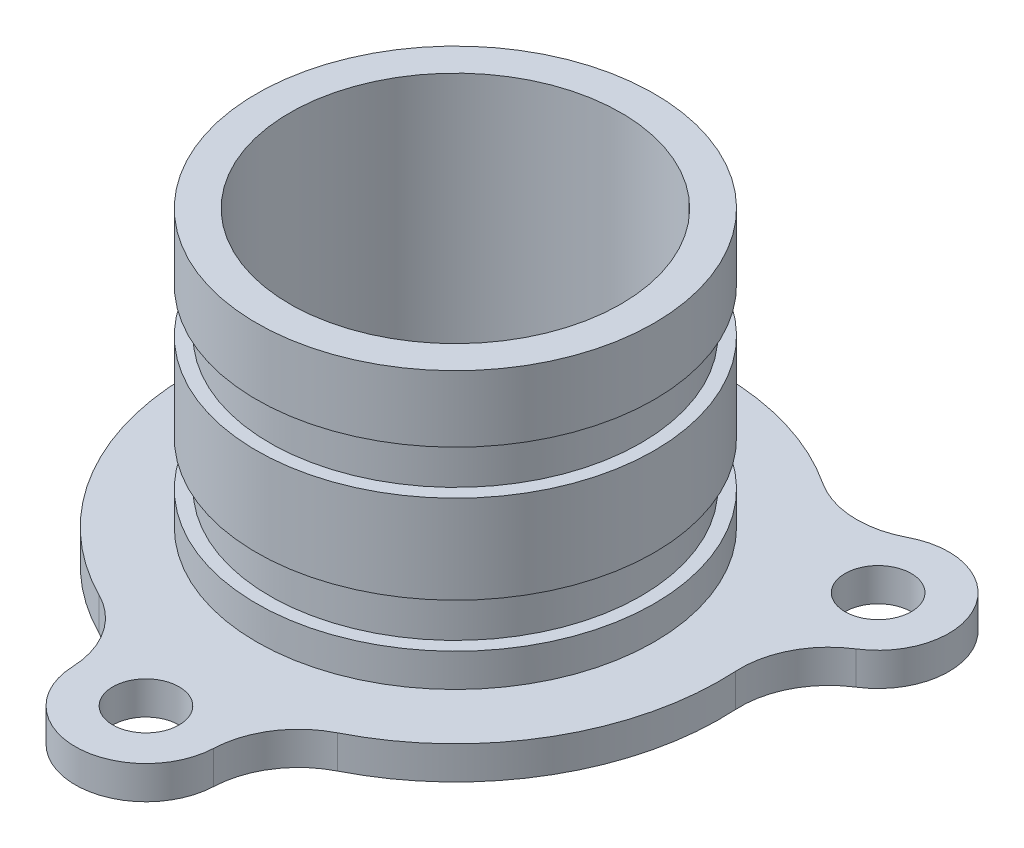
ISO-10303-21;
HEADER;
FILE_DESCRIPTION(('STEP AP214'),'2;1');
FILE_NAME('part.step','',(''),(''),'','','');
FILE_SCHEMA(('AUTOMOTIVE_DESIGN { 1 0 10303 214 1 1 1 1 }'));
ENDSEC;
DATA;
#1=APPLICATION_CONTEXT('core data for automotive mechanical design processes');
#2=APPLICATION_PROTOCOL_DEFINITION('international standard','automotive_design',2000,#1);
#3=PRODUCT_CONTEXT('',#1,'mechanical');
#4=PRODUCT('Part','Part','',(#3));
#5=PRODUCT_RELATED_PRODUCT_CATEGORY('part','',(#4));
#6=PRODUCT_DEFINITION_FORMATION('','',#4);
#7=PRODUCT_DEFINITION_CONTEXT('part definition',#1,'design');
#8=PRODUCT_DEFINITION('design','',#6,#7);
#9=PRODUCT_DEFINITION_SHAPE('','',#8);
#10=(LENGTH_UNIT() NAMED_UNIT(*) SI_UNIT(.MILLI.,.METRE.));
#11=(NAMED_UNIT(*) PLANE_ANGLE_UNIT() SI_UNIT($,.RADIAN.));
#12=(NAMED_UNIT(*) SI_UNIT($,.STERADIAN.) SOLID_ANGLE_UNIT());
#13=UNCERTAINTY_MEASURE_WITH_UNIT(LENGTH_MEASURE(1.E-05),#10,'distance_accuracy_value','');
#14=(GEOMETRIC_REPRESENTATION_CONTEXT(3) GLOBAL_UNCERTAINTY_ASSIGNED_CONTEXT((#13)) GLOBAL_UNIT_ASSIGNED_CONTEXT((#10,
#11,#12)) REPRESENTATION_CONTEXT('',''));
#15=CARTESIAN_POINT('',(0.,0.,0.));
#16=DIRECTION('',(0.,0.,1.));
#17=DIRECTION('',(1.,0.,0.));
#18=AXIS2_PLACEMENT_3D('',#15,#16,#17);
#19=CARTESIAN_POINT('',(45.,70.,0.));
#20=DIRECTION('',(0.,1.,0.));
#21=DIRECTION('',(-1.,0.,0.));
#22=AXIS2_PLACEMENT_3D('',#19,#20,#21);
#23=PLANE('',#22);
#24=CARTESIAN_POINT('',(0.,70.,0.));
#25=DIRECTION('',(0.,-1.,0.));
#26=DIRECTION('',(1.,0.,0.));
#27=AXIS2_PLACEMENT_3D('',#24,#25,#26);
#28=CIRCLE('',#27,37.5);
#29=CARTESIAN_POINT('',(37.5,70.,0.));
#30=VERTEX_POINT('',#29);
#31=EDGE_CURVE('E50',#30,#30,#28,.T.);
#32=ORIENTED_EDGE('',*,*,#31,.T.);
#33=EDGE_LOOP('',(#32));
#34=FACE_BOUND('',#33,.T.);
#35=CARTESIAN_POINT('',(0.,70.,0.));
#36=DIRECTION('',(0.,-1.,0.));
#37=DIRECTION('',(1.,0.,0.));
#38=AXIS2_PLACEMENT_3D('',#35,#36,#37);
#39=CIRCLE('',#38,45.);
#40=CARTESIAN_POINT('',(45.,70.,0.));
#41=VERTEX_POINT('',#40);
#42=EDGE_CURVE('E196',#41,#41,#39,.T.);
#43=ORIENTED_EDGE('',*,*,#42,.F.);
#44=EDGE_LOOP('',(#43));
#45=FACE_BOUND('',#44,.T.);
#46=ADVANCED_FACE('F39',(#34,#45),#23,.T.);
#47=CARTESIAN_POINT('',(0.,-100.894385011522,0.));
#48=DIRECTION('',(0.,-1.,0.));
#49=DIRECTION('',(1.,0.,0.));
#50=AXIS2_PLACEMENT_3D('',#47,#48,#49);
#51=CYLINDRICAL_SURFACE('',#50,37.5);
#52=ORIENTED_EDGE('',*,*,#31,.F.);
#53=EDGE_LOOP('',(#52));
#54=FACE_BOUND('',#53,.T.);
#55=CARTESIAN_POINT('',(0.,0.,0.));
#56=DIRECTION('',(0.,-1.,0.));
#57=DIRECTION('',(1.,0.,0.));
#58=AXIS2_PLACEMENT_3D('',#55,#56,#57);
#59=CIRCLE('',#58,37.5);
#60=CARTESIAN_POINT('',(37.5,0.,0.));
#61=VERTEX_POINT('',#60);
#62=EDGE_CURVE('E244',#61,#61,#59,.T.);
#63=ORIENTED_EDGE('',*,*,#62,.T.);
#64=EDGE_LOOP('',(#63));
#65=FACE_BOUND('',#64,.T.);
#66=ADVANCED_FACE('F247',(#54,#65),#51,.F.);
#67=CARTESIAN_POINT('',(45.,0.,0.));
#68=DIRECTION('',(0.,-1.,0.));
#69=DIRECTION('',(1.,0.,0.));
#70=AXIS2_PLACEMENT_3D('',#67,#68,#69);
#71=PLANE('',#70);
#72=ORIENTED_EDGE('',*,*,#62,.F.);
#73=EDGE_LOOP('',(#72));
#74=FACE_BOUND('',#73,.T.);
#75=CARTESIAN_POINT('',(-60.6650795351003,0.,-35.0249999999994));
#76=DIRECTION('',(0.,-1.,0.));
#77=DIRECTION('',(1.,0.,0.));
#78=AXIS2_PLACEMENT_3D('',#75,#76,#77);
#79=CIRCLE('',#78,7.5);
#80=CARTESIAN_POINT('',(-53.1650795351003,0.,-35.0249999999994));
#81=VERTEX_POINT('',#80);
#82=EDGE_CURVE('E265',#81,#81,#79,.T.);
#83=ORIENTED_EDGE('',*,*,#82,.F.);
#84=EDGE_LOOP('',(#83));
#85=FACE_BOUND('',#84,.T.);
#86=CARTESIAN_POINT('',(60.6650795350998,0.,-35.0250000000003));
#87=DIRECTION('',(0.,-1.,0.));
#88=DIRECTION('',(1.,0.,0.));
#89=AXIS2_PLACEMENT_3D('',#86,#87,#88);
#90=CIRCLE('',#89,7.50000000000001);
#91=CARTESIAN_POINT('',(68.1650795350998,0.,-35.0250000000003));
#92=VERTEX_POINT('',#91);
#93=EDGE_CURVE('E266',#92,#92,#90,.T.);
#94=ORIENTED_EDGE('',*,*,#93,.F.);
#95=EDGE_LOOP('',(#94));
#96=FACE_BOUND('',#95,.T.);
#97=CARTESIAN_POINT('',(0.,0.,70.05));
#98=DIRECTION('',(0.,-1.,0.));
#99=DIRECTION('',(1.,0.,0.));
#100=AXIS2_PLACEMENT_3D('',#97,#98,#99);
#101=CIRCLE('',#100,7.5);
#102=CARTESIAN_POINT('',(7.5,0.,70.05));
#103=VERTEX_POINT('',#102);
#104=EDGE_CURVE('E269',#103,#103,#101,.T.);
#105=ORIENTED_EDGE('',*,*,#104,.F.);
#106=EDGE_LOOP('',(#105));
#107=FACE_BOUND('',#106,.T.);
#108=CARTESIAN_POINT('',(-35.9702505845438,0.,71.5132405424697));
#109=DIRECTION('',(0.,1.,0.));
#110=DIRECTION('',(-1.,0.,0.));
#111=AXIS2_PLACEMENT_3D('',#108,#109,#110);
#112=CIRCLE('',#111,20.);
#113=CARTESIAN_POINT('',(-15.986778037575,0.,70.7003291299865));
#114=VERTEX_POINT('',#113);
#115=CARTESIAN_POINT('',(-26.983304779536,0.,53.6460973713342));
#116=VERTEX_POINT('',#115);
#117=EDGE_CURVE('E165',#114,#116,#112,.T.);
#118=ORIENTED_EDGE('',*,*,#117,.T.);
#119=CARTESIAN_POINT('',(0.,0.,0.));
#120=DIRECTION('',(0.,-1.,0.));
#121=DIRECTION('',(1.,0.,0.));
#122=AXIS2_PLACEMENT_3D('',#119,#120,#121);
#123=CIRCLE('',#122,60.05);
#124=CARTESIAN_POINT('',(-59.950535527237,0.,-3.45482126853093));
#125=VERTEX_POINT('',#124);
#126=EDGE_CURVE('E164',#116,#125,#123,.T.);
#127=ORIENTED_EDGE('',*,*,#126,.T.);
#128=CARTESIAN_POINT('',(-79.9174083089979,0.,-4.60546948452791));
#129=DIRECTION('',(0.,1.,0.));
#130=DIRECTION('',(1.,0.,0.));
#131=AXIS2_PLACEMENT_3D('',#128,#129,#130);
#132=CIRCLE('',#131,20.);
#133=CARTESIAN_POINT('',(-69.2216701012772,0.,-21.5052086597896));
#134=VERTEX_POINT('',#133);
#135=EDGE_CURVE('E166',#125,#134,#132,.T.);
#136=ORIENTED_EDGE('',*,*,#135,.T.);
#137=CARTESIAN_POINT('',(-60.6650795351003,0.,-35.0249999999994));
#138=DIRECTION('',(0.,-1.,0.));
#139=DIRECTION('',(1.,0.,0.));
#140=AXIS2_PLACEMENT_3D('',#137,#138,#139);
#141=CIRCLE('',#140,16.);
#142=CARTESIAN_POINT('',(-53.2348920637018,0.,-49.1951204701964));
#143=VERTEX_POINT('',#142);
#144=EDGE_CURVE('E174',#134,#143,#141,.T.);
#145=ORIENTED_EDGE('',*,*,#144,.T.);
#146=CARTESIAN_POINT('',(-43.9471577244541,0.,-66.9077710579418));
#147=DIRECTION('',(0.,1.,0.));
#148=DIRECTION('',(-1.,0.,0.));
#149=AXIS2_PLACEMENT_3D('',#146,#147,#148);
#150=CIRCLE('',#149,20.);
#151=CARTESIAN_POINT('',(-32.9672307477011,0.,-50.1912761028033));
#152=VERTEX_POINT('',#151);
#153=EDGE_CURVE('E171',#143,#152,#150,.T.);
#154=ORIENTED_EDGE('',*,*,#153,.T.);
#155=CARTESIAN_POINT('',(0.,0.,0.));
#156=DIRECTION('',(0.,-1.,0.));
#157=DIRECTION('',(1.,0.,0.));
#158=AXIS2_PLACEMENT_3D('',#155,#156,#157);
#159=CIRCLE('',#158,60.05);
#160=CARTESIAN_POINT('',(32.9672307477011,0.,-50.1912761028033));
#161=VERTEX_POINT('',#160);
#162=EDGE_CURVE('E178',#152,#161,#159,.T.);
#163=ORIENTED_EDGE('',*,*,#162,.T.);
#164=CARTESIAN_POINT('',(43.9471577244538,0.,-66.907771057942));
#165=DIRECTION('',(0.,1.,0.));
#166=DIRECTION('',(1.,0.,0.));
#167=AXIS2_PLACEMENT_3D('',#164,#165,#166);
#168=CIRCLE('',#167,20.);
#169=CARTESIAN_POINT('',(53.2348920637016,0.,-49.1951204701966));
#170=VERTEX_POINT('',#169);
#171=EDGE_CURVE('E182',#161,#170,#168,.T.);
#172=ORIENTED_EDGE('',*,*,#171,.T.);
#173=CARTESIAN_POINT('',(60.6650795350998,0.,-35.0250000000003));
#174=DIRECTION('',(0.,-1.,0.));
#175=DIRECTION('',(1.,0.,0.));
#176=AXIS2_PLACEMENT_3D('',#173,#174,#175);
#177=CIRCLE('',#176,16.);
#178=CARTESIAN_POINT('',(69.2216701012767,0.,-21.5052086597905));
#179=VERTEX_POINT('',#178);
#180=EDGE_CURVE('E184',#170,#179,#177,.T.);
#181=ORIENTED_EDGE('',*,*,#180,.T.);
#182=CARTESIAN_POINT('',(79.9174083089979,0.,-4.60546948452819));
#183=DIRECTION('',(0.,1.,0.));
#184=DIRECTION('',(-1.,0.,0.));
#185=AXIS2_PLACEMENT_3D('',#182,#183,#184);
#186=CIRCLE('',#185,20.);
#187=CARTESIAN_POINT('',(59.950535527237,0.,-3.45482126853086));
#188=VERTEX_POINT('',#187);
#189=EDGE_CURVE('E189',#179,#188,#186,.T.);
#190=ORIENTED_EDGE('',*,*,#189,.T.);
#191=CARTESIAN_POINT('',(0.,0.,0.));
#192=DIRECTION('',(0.,-1.,0.));
#193=DIRECTION('',(1.,0.,0.));
#194=AXIS2_PLACEMENT_3D('',#191,#192,#193);
#195=CIRCLE('',#194,60.05);
#196=CARTESIAN_POINT('',(26.983304779536,0.,53.6460973713342));
#197=VERTEX_POINT('',#196);
#198=EDGE_CURVE('E186',#188,#197,#195,.T.);
#199=ORIENTED_EDGE('',*,*,#198,.T.);
#200=CARTESIAN_POINT('',(35.9702505845438,0.,71.5132405424697));
#201=DIRECTION('',(0.,1.,0.));
#202=DIRECTION('',(1.,0.,0.));
#203=AXIS2_PLACEMENT_3D('',#200,#201,#202);
#204=CIRCLE('',#203,20.);
#205=CARTESIAN_POINT('',(15.986778037575,0.,70.7003291299865));
#206=VERTEX_POINT('',#205);
#207=EDGE_CURVE('E137',#197,#206,#204,.T.);
#208=ORIENTED_EDGE('',*,*,#207,.T.);
#209=CARTESIAN_POINT('',(0.,0.,70.05));
#210=DIRECTION('',(0.,-1.,0.));
#211=DIRECTION('',(1.,0.,0.));
#212=AXIS2_PLACEMENT_3D('',#209,#210,#211);
#213=CIRCLE('',#212,16.);
#214=EDGE_CURVE('E193',#206,#114,#213,.T.);
#215=ORIENTED_EDGE('',*,*,#214,.T.);
#216=EDGE_LOOP('',(#118,#127,#136,#145,#154,#163,#172,#181,#190,#199,#208,#215));
#217=FACE_BOUND('',#216,.T.);
#218=ADVANCED_FACE('F252',(#74,#85,#96,#107,#217),#71,.T.);
#219=CARTESIAN_POINT('',(0.,-100.894385011522,0.));
#220=DIRECTION('',(0.,-1.,0.));
#221=DIRECTION('',(1.,0.,0.));
#222=AXIS2_PLACEMENT_3D('',#219,#220,#221);
#223=CYLINDRICAL_SURFACE('',#222,45.);
#224=CARTESIAN_POINT('',(0.,7.49999999999999,0.));
#225=DIRECTION('',(0.,1.,0.));
#226=DIRECTION('',(-1.,0.,0.));
#227=AXIS2_PLACEMENT_3D('',#224,#225,#226);
#228=CIRCLE('',#227,45.);
#229=CARTESIAN_POINT('',(-45.,7.49999999999998,0.));
#230=VERTEX_POINT('',#229);
#231=EDGE_CURVE('E11',#230,#230,#228,.F.);
#232=ORIENTED_EDGE('',*,*,#231,.F.);
#233=EDGE_LOOP('',(#232));
#234=FACE_BOUND('',#233,.T.);
#235=CARTESIAN_POINT('',(0.,15.,0.));
#236=DIRECTION('',(0.,-1.,0.));
#237=DIRECTION('',(1.,0.,0.));
#238=AXIS2_PLACEMENT_3D('',#235,#236,#237);
#239=CIRCLE('',#238,45.);
#240=CARTESIAN_POINT('',(45.,15.,0.));
#241=VERTEX_POINT('',#240);
#242=EDGE_CURVE('E239',#241,#241,#239,.T.);
#243=ORIENTED_EDGE('',*,*,#242,.T.);
#244=EDGE_LOOP('',(#243));
#245=FACE_BOUND('',#244,.T.);
#246=ADVANCED_FACE('F260',(#234,#245),#223,.T.);
#247=CARTESIAN_POINT('',(45.,15.,0.));
#248=DIRECTION('',(0.,1.,0.));
#249=DIRECTION('',(-1.,0.,0.));
#250=AXIS2_PLACEMENT_3D('',#247,#248,#249);
#251=PLANE('',#250);
#252=CARTESIAN_POINT('',(0.,15.,0.));
#253=DIRECTION('',(0.,-1.,0.));
#254=DIRECTION('',(1.,0.,0.));
#255=AXIS2_PLACEMENT_3D('',#252,#253,#254);
#256=CIRCLE('',#255,42.);
#257=CARTESIAN_POINT('',(42.,15.,0.));
#258=VERTEX_POINT('',#257);
#259=EDGE_CURVE('E237',#258,#258,#256,.T.);
#260=ORIENTED_EDGE('',*,*,#259,.T.);
#261=EDGE_LOOP('',(#260));
#262=FACE_BOUND('',#261,.T.);
#263=ORIENTED_EDGE('',*,*,#242,.F.);
#264=EDGE_LOOP('',(#263));
#265=FACE_BOUND('',#264,.T.);
#266=ADVANCED_FACE('F328',(#262,#265),#251,.T.);
#267=CARTESIAN_POINT('',(0.,-100.894385011522,0.));
#268=DIRECTION('',(0.,-1.,0.));
#269=DIRECTION('',(1.,0.,0.));
#270=AXIS2_PLACEMENT_3D('',#267,#268,#269);
#271=CYLINDRICAL_SURFACE('',#270,42.);
#272=CARTESIAN_POINT('',(0.,25.,0.));
#273=DIRECTION('',(0.,-1.,0.));
#274=DIRECTION('',(1.,0.,0.));
#275=AXIS2_PLACEMENT_3D('',#272,#273,#274);
#276=CIRCLE('',#275,42.);
#277=CARTESIAN_POINT('',(42.,25.,0.));
#278=VERTEX_POINT('',#277);
#279=EDGE_CURVE('E233',#278,#278,#276,.T.);
#280=ORIENTED_EDGE('',*,*,#279,.T.);
#281=EDGE_LOOP('',(#280));
#282=FACE_BOUND('',#281,.T.);
#283=ORIENTED_EDGE('',*,*,#259,.F.);
#284=EDGE_LOOP('',(#283));
#285=FACE_BOUND('',#284,.T.);
#286=ADVANCED_FACE('F334',(#282,#285),#271,.T.);
#287=CARTESIAN_POINT('',(42.,25.,0.));
#288=DIRECTION('',(0.,-1.,0.));
#289=DIRECTION('',(1.,0.,0.));
#290=AXIS2_PLACEMENT_3D('',#287,#288,#289);
#291=PLANE('',#290);
#292=CARTESIAN_POINT('',(0.,25.,0.));
#293=DIRECTION('',(0.,-1.,0.));
#294=DIRECTION('',(1.,0.,0.));
#295=AXIS2_PLACEMENT_3D('',#292,#293,#294);
#296=CIRCLE('',#295,45.);
#297=CARTESIAN_POINT('',(45.,25.,0.));
#298=VERTEX_POINT('',#297);
#299=EDGE_CURVE('E226',#298,#298,#296,.T.);
#300=ORIENTED_EDGE('',*,*,#299,.T.);
#301=EDGE_LOOP('',(#300));
#302=FACE_BOUND('',#301,.T.);
#303=ORIENTED_EDGE('',*,*,#279,.F.);
#304=EDGE_LOOP('',(#303));
#305=FACE_BOUND('',#304,.T.);
#306=ADVANCED_FACE('F343',(#302,#305),#291,.T.);
#307=CARTESIAN_POINT('',(0.,-100.894385011522,0.));
#308=DIRECTION('',(0.,-1.,0.));
#309=DIRECTION('',(1.,0.,0.));
#310=AXIS2_PLACEMENT_3D('',#307,#308,#309);
#311=CYLINDRICAL_SURFACE('',#310,45.);
#312=CARTESIAN_POINT('',(0.,45.,0.));
#313=DIRECTION('',(0.,-1.,0.));
#314=DIRECTION('',(1.,0.,0.));
#315=AXIS2_PLACEMENT_3D('',#312,#313,#314);
#316=CIRCLE('',#315,45.);
#317=CARTESIAN_POINT('',(45.,45.,0.));
#318=VERTEX_POINT('',#317);
#319=EDGE_CURVE('E229',#318,#318,#316,.T.);
#320=ORIENTED_EDGE('',*,*,#319,.T.);
#321=EDGE_LOOP('',(#320));
#322=FACE_BOUND('',#321,.T.);
#323=ORIENTED_EDGE('',*,*,#299,.F.);
#324=EDGE_LOOP('',(#323));
#325=FACE_BOUND('',#324,.T.);
#326=ADVANCED_FACE('F354',(#322,#325),#311,.T.);
#327=CARTESIAN_POINT('',(45.,45.,0.));
#328=DIRECTION('',(0.,1.,0.));
#329=DIRECTION('',(-1.,0.,0.));
#330=AXIS2_PLACEMENT_3D('',#327,#328,#329);
#331=PLANE('',#330);
#332=CARTESIAN_POINT('',(0.,45.,0.));
#333=DIRECTION('',(0.,-1.,0.));
#334=DIRECTION('',(1.,0.,0.));
#335=AXIS2_PLACEMENT_3D('',#332,#333,#334);
#336=CIRCLE('',#335,42.);
#337=CARTESIAN_POINT('',(42.,45.,0.));
#338=VERTEX_POINT('',#337);
#339=EDGE_CURVE('E221',#338,#338,#336,.T.);
#340=ORIENTED_EDGE('',*,*,#339,.T.);
#341=EDGE_LOOP('',(#340));
#342=FACE_BOUND('',#341,.T.);
#343=ORIENTED_EDGE('',*,*,#319,.F.);
#344=EDGE_LOOP('',(#343));
#345=FACE_BOUND('',#344,.T.);
#346=ADVANCED_FACE('F363',(#342,#345),#331,.T.);
#347=CARTESIAN_POINT('',(0.,-100.894385011522,0.));
#348=DIRECTION('',(0.,-1.,0.));
#349=DIRECTION('',(1.,0.,0.));
#350=AXIS2_PLACEMENT_3D('',#347,#348,#349);
#351=CYLINDRICAL_SURFACE('',#350,42.);
#352=CARTESIAN_POINT('',(0.,55.,0.));
#353=DIRECTION('',(0.,-1.,0.));
#354=DIRECTION('',(1.,0.,0.));
#355=AXIS2_PLACEMENT_3D('',#352,#353,#354);
#356=CIRCLE('',#355,42.);
#357=CARTESIAN_POINT('',(42.,55.,0.));
#358=VERTEX_POINT('',#357);
#359=EDGE_CURVE('E222',#358,#358,#356,.T.);
#360=ORIENTED_EDGE('',*,*,#359,.T.);
#361=EDGE_LOOP('',(#360));
#362=FACE_BOUND('',#361,.T.);
#363=ORIENTED_EDGE('',*,*,#339,.F.);
#364=EDGE_LOOP('',(#363));
#365=FACE_BOUND('',#364,.T.);
#366=ADVANCED_FACE('F367',(#362,#365),#351,.T.);
#367=CARTESIAN_POINT('',(42.,55.,0.));
#368=DIRECTION('',(0.,-1.,0.));
#369=DIRECTION('',(1.,0.,0.));
#370=AXIS2_PLACEMENT_3D('',#367,#368,#369);
#371=PLANE('',#370);
#372=CARTESIAN_POINT('',(0.,55.,0.));
#373=DIRECTION('',(0.,-1.,0.));
#374=DIRECTION('',(1.,0.,0.));
#375=AXIS2_PLACEMENT_3D('',#372,#373,#374);
#376=CIRCLE('',#375,45.);
#377=CARTESIAN_POINT('',(45.,55.,0.));
#378=VERTEX_POINT('',#377);
#379=EDGE_CURVE('E217',#378,#378,#376,.T.);
#380=ORIENTED_EDGE('',*,*,#379,.T.);
#381=EDGE_LOOP('',(#380));
#382=FACE_BOUND('',#381,.T.);
#383=ORIENTED_EDGE('',*,*,#359,.F.);
#384=EDGE_LOOP('',(#383));
#385=FACE_BOUND('',#384,.T.);
#386=ADVANCED_FACE('F377',(#382,#385),#371,.T.);
#387=CARTESIAN_POINT('',(0.,-100.894385011522,0.));
#388=DIRECTION('',(0.,-1.,0.));
#389=DIRECTION('',(1.,0.,0.));
#390=AXIS2_PLACEMENT_3D('',#387,#388,#389);
#391=CYLINDRICAL_SURFACE('',#390,45.);
#392=ORIENTED_EDGE('',*,*,#42,.T.);
#393=EDGE_LOOP('',(#392));
#394=FACE_BOUND('',#393,.T.);
#395=ORIENTED_EDGE('',*,*,#379,.F.);
#396=EDGE_LOOP('',(#395));
#397=FACE_BOUND('',#396,.T.);
#398=ADVANCED_FACE('F318',(#394,#397),#391,.T.);
#399=CARTESIAN_POINT('',(-35.9702505845438,7.49999999999999,71.5132405424697));
#400=DIRECTION('',(0.,-1.,0.));
#401=DIRECTION('',(1.,0.,0.));
#402=AXIS2_PLACEMENT_3D('',#399,#400,#401);
#403=CYLINDRICAL_SURFACE('',#402,20.);
#404=ORIENTED_EDGE('',*,*,#117,.F.);
#405=DIRECTION('',(0.,-1.,0.));
#406=VECTOR('',#405,1.);
#407=CARTESIAN_POINT('',(-15.986778037575,7.5,70.7003291299865));
#408=LINE('',#407,#406);
#409=CARTESIAN_POINT('',(-15.986778037575,7.5,70.7003291299865));
#410=VERTEX_POINT('',#409);
#411=EDGE_CURVE('E54',#410,#114,#408,.T.);
#412=ORIENTED_EDGE('',*,*,#411,.F.);
#413=CARTESIAN_POINT('',(-35.9702505845438,7.49999999999999,71.5132405424697));
#414=DIRECTION('',(0.,1.,0.));
#415=DIRECTION('',(-1.,0.,0.));
#416=AXIS2_PLACEMENT_3D('',#413,#414,#415);
#417=CIRCLE('',#416,20.);
#418=CARTESIAN_POINT('',(-26.983304779536,7.49999999999999,53.6460973713342));
#419=VERTEX_POINT('',#418);
#420=EDGE_CURVE('E198',#410,#419,#417,.T.);
#421=ORIENTED_EDGE('',*,*,#420,.T.);
#422=DIRECTION('',(0.,-1.,0.));
#423=VECTOR('',#422,1.);
#424=CARTESIAN_POINT('',(-26.983304779536,7.49999999999999,53.6460973713342));
#425=LINE('',#424,#423);
#426=EDGE_CURVE('E107',#419,#116,#425,.T.);
#427=ORIENTED_EDGE('',*,*,#426,.T.);
#428=EDGE_LOOP('',(#404,#412,#421,#427));
#429=FACE_BOUND('',#428,.T.);
#430=ADVANCED_FACE('F271',(#429),#403,.F.);
#431=CARTESIAN_POINT('',(0.,7.5,70.05));
#432=DIRECTION('',(0.,-1.,0.));
#433=DIRECTION('',(1.,0.,0.));
#434=AXIS2_PLACEMENT_3D('',#431,#432,#433);
#435=CYLINDRICAL_SURFACE('',#434,16.);
#436=ORIENTED_EDGE('',*,*,#214,.F.);
#437=DIRECTION('',(0.,-1.,0.));
#438=VECTOR('',#437,1.);
#439=CARTESIAN_POINT('',(15.986778037575,7.5,70.7003291299865));
#440=LINE('',#439,#438);
#441=CARTESIAN_POINT('',(15.986778037575,7.5,70.7003291299865));
#442=VERTEX_POINT('',#441);
#443=EDGE_CURVE('E96',#442,#206,#440,.T.);
#444=ORIENTED_EDGE('',*,*,#443,.F.);
#445=CARTESIAN_POINT('',(0.,7.5,70.05));
#446=DIRECTION('',(0.,-1.,0.));
#447=DIRECTION('',(1.,0.,0.));
#448=AXIS2_PLACEMENT_3D('',#445,#446,#447);
#449=CIRCLE('',#448,16.);
#450=EDGE_CURVE('E155',#442,#410,#449,.T.);
#451=ORIENTED_EDGE('',*,*,#450,.T.);
#452=ORIENTED_EDGE('',*,*,#411,.T.);
#453=EDGE_LOOP('',(#436,#444,#451,#452));
#454=FACE_BOUND('',#453,.T.);
#455=ADVANCED_FACE('F309',(#454),#435,.T.);
#456=CARTESIAN_POINT('',(35.9702505845438,7.50000000000001,71.5132405424697));
#457=DIRECTION('',(0.,-1.,0.));
#458=DIRECTION('',(1.,0.,0.));
#459=AXIS2_PLACEMENT_3D('',#456,#457,#458);
#460=CYLINDRICAL_SURFACE('',#459,20.);
#461=ORIENTED_EDGE('',*,*,#207,.F.);
#462=DIRECTION('',(0.,-1.,0.));
#463=VECTOR('',#462,1.);
#464=CARTESIAN_POINT('',(26.983304779536,7.50000000000001,53.6460973713342));
#465=LINE('',#464,#463);
#466=CARTESIAN_POINT('',(26.983304779536,7.50000000000001,53.6460973713342));
#467=VERTEX_POINT('',#466);
#468=EDGE_CURVE('E135',#467,#197,#465,.T.);
#469=ORIENTED_EDGE('',*,*,#468,.F.);
#470=CARTESIAN_POINT('',(35.9702505845438,7.50000000000001,71.5132405424697));
#471=DIRECTION('',(0.,1.,0.));
#472=DIRECTION('',(1.,0.,0.));
#473=AXIS2_PLACEMENT_3D('',#470,#471,#472);
#474=CIRCLE('',#473,20.);
#475=EDGE_CURVE('E140',#467,#442,#474,.T.);
#476=ORIENTED_EDGE('',*,*,#475,.T.);
#477=ORIENTED_EDGE('',*,*,#443,.T.);
#478=EDGE_LOOP('',(#461,#469,#476,#477));
#479=FACE_BOUND('',#478,.T.);
#480=ADVANCED_FACE('F136',(#479),#460,.F.);
#481=CARTESIAN_POINT('',(0.,7.5,0.));
#482=DIRECTION('',(0.,-1.,0.));
#483=DIRECTION('',(1.,0.,0.));
#484=AXIS2_PLACEMENT_3D('',#481,#482,#483);
#485=CYLINDRICAL_SURFACE('',#484,60.05);
#486=ORIENTED_EDGE('',*,*,#198,.F.);
#487=DIRECTION('',(0.,-1.,0.));
#488=VECTOR('',#487,1.);
#489=CARTESIAN_POINT('',(59.950535527237,7.50000000000001,-3.45482126853086));
#490=LINE('',#489,#488);
#491=CARTESIAN_POINT('',(59.950535527237,7.50000000000001,-3.45482126853086));
#492=VERTEX_POINT('',#491);
#493=EDGE_CURVE('E145',#492,#188,#490,.T.);
#494=ORIENTED_EDGE('',*,*,#493,.F.);
#495=CARTESIAN_POINT('',(0.,7.5,0.));
#496=DIRECTION('',(0.,-1.,0.));
#497=DIRECTION('',(1.,0.,0.));
#498=AXIS2_PLACEMENT_3D('',#495,#496,#497);
#499=CIRCLE('',#498,60.05);
#500=EDGE_CURVE('E147',#492,#467,#499,.T.);
#501=ORIENTED_EDGE('',*,*,#500,.T.);
#502=ORIENTED_EDGE('',*,*,#468,.T.);
#503=EDGE_LOOP('',(#486,#494,#501,#502));
#504=FACE_BOUND('',#503,.T.);
#505=ADVANCED_FACE('F152',(#504),#485,.T.);
#506=CARTESIAN_POINT('',(79.9174083089979,7.50000000000001,-4.60546948452819));
#507=DIRECTION('',(0.,-1.,0.));
#508=DIRECTION('',(1.,0.,0.));
#509=AXIS2_PLACEMENT_3D('',#506,#507,#508);
#510=CYLINDRICAL_SURFACE('',#509,20.);
#511=ORIENTED_EDGE('',*,*,#189,.F.);
#512=DIRECTION('',(0.,-1.,0.));
#513=VECTOR('',#512,1.);
#514=CARTESIAN_POINT('',(69.2216701012767,7.50000000000001,-21.5052086597905));
#515=LINE('',#514,#513);
#516=CARTESIAN_POINT('',(69.2216701012767,7.50000000000001,-21.5052086597905));
#517=VERTEX_POINT('',#516);
#518=EDGE_CURVE('E203',#517,#179,#515,.T.);
#519=ORIENTED_EDGE('',*,*,#518,.F.);
#520=CARTESIAN_POINT('',(79.9174083089979,7.50000000000001,-4.60546948452819));
#521=DIRECTION('',(0.,1.,0.));
#522=DIRECTION('',(-1.,0.,0.));
#523=AXIS2_PLACEMENT_3D('',#520,#521,#522);
#524=CIRCLE('',#523,20.);
#525=EDGE_CURVE('E154',#517,#492,#524,.T.);
#526=ORIENTED_EDGE('',*,*,#525,.T.);
#527=ORIENTED_EDGE('',*,*,#493,.T.);
#528=EDGE_LOOP('',(#511,#519,#526,#527));
#529=FACE_BOUND('',#528,.T.);
#530=ADVANCED_FACE('F310',(#529),#510,.F.);
#531=CARTESIAN_POINT('',(60.6650795350998,7.50000000000001,-35.0250000000003));
#532=DIRECTION('',(0.,-1.,0.));
#533=DIRECTION('',(1.,0.,0.));
#534=AXIS2_PLACEMENT_3D('',#531,#532,#533);
#535=CYLINDRICAL_SURFACE('',#534,16.);
#536=ORIENTED_EDGE('',*,*,#180,.F.);
#537=DIRECTION('',(0.,-1.,0.));
#538=VECTOR('',#537,1.);
#539=CARTESIAN_POINT('',(53.2348920637016,7.50000000000001,-49.1951204701966));
#540=LINE('',#539,#538);
#541=CARTESIAN_POINT('',(53.2348920637016,7.50000000000001,-49.1951204701966));
#542=VERTEX_POINT('',#541);
#543=EDGE_CURVE('E201',#542,#170,#540,.T.);
#544=ORIENTED_EDGE('',*,*,#543,.F.);
#545=CARTESIAN_POINT('',(60.6650795350998,7.50000000000001,-35.0250000000003));
#546=DIRECTION('',(0.,-1.,0.));
#547=DIRECTION('',(1.,0.,0.));
#548=AXIS2_PLACEMENT_3D('',#545,#546,#547);
#549=CIRCLE('',#548,16.);
#550=EDGE_CURVE('E160',#542,#517,#549,.T.);
#551=ORIENTED_EDGE('',*,*,#550,.T.);
#552=ORIENTED_EDGE('',*,*,#518,.T.);
#553=EDGE_LOOP('',(#536,#544,#551,#552));
#554=FACE_BOUND('',#553,.T.);
#555=ADVANCED_FACE('F308',(#554),#535,.T.);
#556=CARTESIAN_POINT('',(43.9471577244538,7.50000000000001,-66.907771057942));
#557=DIRECTION('',(0.,-1.,0.));
#558=DIRECTION('',(1.,0.,0.));
#559=AXIS2_PLACEMENT_3D('',#556,#557,#558);
#560=CYLINDRICAL_SURFACE('',#559,20.);
#561=ORIENTED_EDGE('',*,*,#171,.F.);
#562=DIRECTION('',(0.,-1.,0.));
#563=VECTOR('',#562,1.);
#564=CARTESIAN_POINT('',(32.9672307477011,7.50000000000001,-50.1912761028033));
#565=LINE('',#564,#563);
#566=CARTESIAN_POINT('',(32.9672307477011,7.50000000000001,-50.1912761028033));
#567=VERTEX_POINT('',#566);
#568=EDGE_CURVE('E202',#567,#161,#565,.T.);
#569=ORIENTED_EDGE('',*,*,#568,.F.);
#570=CARTESIAN_POINT('',(43.9471577244538,7.50000000000001,-66.907771057942));
#571=DIRECTION('',(0.,1.,0.));
#572=DIRECTION('',(1.,0.,0.));
#573=AXIS2_PLACEMENT_3D('',#570,#571,#572);
#574=CIRCLE('',#573,20.);
#575=EDGE_CURVE('E305',#567,#542,#574,.T.);
#576=ORIENTED_EDGE('',*,*,#575,.T.);
#577=ORIENTED_EDGE('',*,*,#543,.T.);
#578=EDGE_LOOP('',(#561,#569,#576,#577));
#579=FACE_BOUND('',#578,.T.);
#580=ADVANCED_FACE('F300',(#579),#560,.F.);
#581=CARTESIAN_POINT('',(0.,7.5,0.));
#582=DIRECTION('',(0.,-1.,0.));
#583=DIRECTION('',(1.,0.,0.));
#584=AXIS2_PLACEMENT_3D('',#581,#582,#583);
#585=CYLINDRICAL_SURFACE('',#584,60.05);
#586=ORIENTED_EDGE('',*,*,#162,.F.);
#587=DIRECTION('',(0.,-1.,0.));
#588=VECTOR('',#587,1.);
#589=CARTESIAN_POINT('',(-32.9672307477011,7.49999999999999,-50.1912761028033));
#590=LINE('',#589,#588);
#591=CARTESIAN_POINT('',(-32.9672307477011,7.49999999999999,-50.1912761028033));
#592=VERTEX_POINT('',#591);
#593=EDGE_CURVE('E210',#592,#152,#590,.T.);
#594=ORIENTED_EDGE('',*,*,#593,.F.);
#595=CARTESIAN_POINT('',(0.,7.5,0.));
#596=DIRECTION('',(0.,-1.,0.));
#597=DIRECTION('',(1.,0.,0.));
#598=AXIS2_PLACEMENT_3D('',#595,#596,#597);
#599=CIRCLE('',#598,60.05);
#600=EDGE_CURVE('E565',#592,#567,#599,.T.);
#601=ORIENTED_EDGE('',*,*,#600,.T.);
#602=ORIENTED_EDGE('',*,*,#568,.T.);
#603=EDGE_LOOP('',(#586,#594,#601,#602));
#604=FACE_BOUND('',#603,.T.);
#605=ADVANCED_FACE('F293',(#604),#585,.T.);
#606=CARTESIAN_POINT('',(-43.9471577244541,7.49999999999999,-66.9077710579418));
#607=DIRECTION('',(0.,-1.,0.));
#608=DIRECTION('',(1.,0.,0.));
#609=AXIS2_PLACEMENT_3D('',#606,#607,#608);
#610=CYLINDRICAL_SURFACE('',#609,20.);
#611=ORIENTED_EDGE('',*,*,#153,.F.);
#612=DIRECTION('',(0.,-1.,0.));
#613=VECTOR('',#612,1.);
#614=CARTESIAN_POINT('',(-53.2348920637018,7.49999999999999,-49.1951204701964));
#615=LINE('',#614,#613);
#616=CARTESIAN_POINT('',(-53.2348920637018,7.49999999999999,-49.1951204701964));
#617=VERTEX_POINT('',#616);
#618=EDGE_CURVE('E207',#617,#143,#615,.T.);
#619=ORIENTED_EDGE('',*,*,#618,.F.);
#620=CARTESIAN_POINT('',(-43.9471577244541,7.49999999999999,-66.9077710579418));
#621=DIRECTION('',(0.,1.,0.));
#622=DIRECTION('',(-1.,0.,0.));
#623=AXIS2_PLACEMENT_3D('',#620,#621,#622);
#624=CIRCLE('',#623,20.);
#625=EDGE_CURVE('E292',#617,#592,#624,.T.);
#626=ORIENTED_EDGE('',*,*,#625,.T.);
#627=ORIENTED_EDGE('',*,*,#593,.T.);
#628=EDGE_LOOP('',(#611,#619,#626,#627));
#629=FACE_BOUND('',#628,.T.);
#630=ADVANCED_FACE('F287',(#629),#610,.F.);
#631=CARTESIAN_POINT('',(-60.6650795351003,7.49999999999999,-35.0249999999994));
#632=DIRECTION('',(0.,-1.,0.));
#633=DIRECTION('',(1.,0.,0.));
#634=AXIS2_PLACEMENT_3D('',#631,#632,#633);
#635=CYLINDRICAL_SURFACE('',#634,16.);
#636=ORIENTED_EDGE('',*,*,#144,.F.);
#637=DIRECTION('',(0.,-1.,0.));
#638=VECTOR('',#637,1.);
#639=CARTESIAN_POINT('',(-69.2216701012772,7.49999999999999,-21.5052086597896));
#640=LINE('',#639,#638);
#641=CARTESIAN_POINT('',(-69.2216701012772,7.49999999999999,-21.5052086597896));
#642=VERTEX_POINT('',#641);
#643=EDGE_CURVE('E211',#642,#134,#640,.T.);
#644=ORIENTED_EDGE('',*,*,#643,.F.);
#645=CARTESIAN_POINT('',(-60.6650795351003,7.49999999999999,-35.0249999999994));
#646=DIRECTION('',(0.,-1.,0.));
#647=DIRECTION('',(1.,0.,0.));
#648=AXIS2_PLACEMENT_3D('',#645,#646,#647);
#649=CIRCLE('',#648,16.);
#650=EDGE_CURVE('E281',#642,#617,#649,.T.);
#651=ORIENTED_EDGE('',*,*,#650,.T.);
#652=ORIENTED_EDGE('',*,*,#618,.T.);
#653=EDGE_LOOP('',(#636,#644,#651,#652));
#654=FACE_BOUND('',#653,.T.);
#655=ADVANCED_FACE('F284',(#654),#635,.T.);
#656=CARTESIAN_POINT('',(-79.9174083089979,7.49999999999998,-4.60546948452791));
#657=DIRECTION('',(0.,-1.,0.));
#658=DIRECTION('',(1.,0.,0.));
#659=AXIS2_PLACEMENT_3D('',#656,#657,#658);
#660=CYLINDRICAL_SURFACE('',#659,20.);
#661=ORIENTED_EDGE('',*,*,#135,.F.);
#662=DIRECTION('',(0.,-1.,0.));
#663=VECTOR('',#662,1.);
#664=CARTESIAN_POINT('',(-59.950535527237,7.49999999999999,-3.45482126853093));
#665=LINE('',#664,#663);
#666=CARTESIAN_POINT('',(-59.950535527237,7.49999999999999,-3.45482126853093));
#667=VERTEX_POINT('',#666);
#668=EDGE_CURVE('E213',#667,#125,#665,.T.);
#669=ORIENTED_EDGE('',*,*,#668,.F.);
#670=CARTESIAN_POINT('',(-79.9174083089979,7.49999999999998,-4.60546948452791));
#671=DIRECTION('',(0.,1.,0.));
#672=DIRECTION('',(1.,0.,0.));
#673=AXIS2_PLACEMENT_3D('',#670,#671,#672);
#674=CIRCLE('',#673,20.);
#675=EDGE_CURVE('E557',#667,#642,#674,.T.);
#676=ORIENTED_EDGE('',*,*,#675,.T.);
#677=ORIENTED_EDGE('',*,*,#643,.T.);
#678=EDGE_LOOP('',(#661,#669,#676,#677));
#679=FACE_BOUND('',#678,.T.);
#680=ADVANCED_FACE('F279',(#679),#660,.F.);
#681=CARTESIAN_POINT('',(0.,7.5,0.));
#682=DIRECTION('',(0.,-1.,0.));
#683=DIRECTION('',(1.,0.,0.));
#684=AXIS2_PLACEMENT_3D('',#681,#682,#683);
#685=CYLINDRICAL_SURFACE('',#684,60.05);
#686=ORIENTED_EDGE('',*,*,#126,.F.);
#687=ORIENTED_EDGE('',*,*,#426,.F.);
#688=CARTESIAN_POINT('',(0.,7.5,0.));
#689=DIRECTION('',(0.,-1.,0.));
#690=DIRECTION('',(1.,0.,0.));
#691=AXIS2_PLACEMENT_3D('',#688,#689,#690);
#692=CIRCLE('',#691,60.05);
#693=EDGE_CURVE('E273',#419,#667,#692,.T.);
#694=ORIENTED_EDGE('',*,*,#693,.T.);
#695=ORIENTED_EDGE('',*,*,#668,.T.);
#696=EDGE_LOOP('',(#686,#687,#694,#695));
#697=FACE_BOUND('',#696,.T.);
#698=ADVANCED_FACE('F275',(#697),#685,.T.);
#699=CARTESIAN_POINT('',(-17.9851252922719,7.5,35.7566202712348));
#700=DIRECTION('',(0.,1.,0.));
#701=DIRECTION('',(-1.,0.,0.));
#702=AXIS2_PLACEMENT_3D('',#699,#700,#701);
#703=PLANE('',#702);
#704=ORIENTED_EDGE('',*,*,#231,.T.);
#705=EDGE_LOOP('',(#704));
#706=FACE_BOUND('',#705,.T.);
#707=CARTESIAN_POINT('',(-60.6650795351003,7.49999999999999,-35.0249999999994));
#708=DIRECTION('',(0.,-1.,0.));
#709=DIRECTION('',(1.,0.,0.));
#710=AXIS2_PLACEMENT_3D('',#707,#708,#709);
#711=CIRCLE('',#710,7.5);
#712=CARTESIAN_POINT('',(-53.1650795351003,7.49999999999999,-35.0249999999994));
#713=VERTEX_POINT('',#712);
#714=EDGE_CURVE('E544',#713,#713,#711,.T.);
#715=ORIENTED_EDGE('',*,*,#714,.T.);
#716=EDGE_LOOP('',(#715));
#717=FACE_BOUND('',#716,.T.);
#718=CARTESIAN_POINT('',(60.6650795350998,7.50000000000001,-35.0250000000003));
#719=DIRECTION('',(0.,-1.,0.));
#720=DIRECTION('',(1.,0.,0.));
#721=AXIS2_PLACEMENT_3D('',#718,#719,#720);
#722=CIRCLE('',#721,7.50000000000001);
#723=CARTESIAN_POINT('',(68.1650795350998,7.50000000000001,-35.0250000000003));
#724=VERTEX_POINT('',#723);
#725=EDGE_CURVE('E548',#724,#724,#722,.T.);
#726=ORIENTED_EDGE('',*,*,#725,.T.);
#727=EDGE_LOOP('',(#726));
#728=FACE_BOUND('',#727,.T.);
#729=CARTESIAN_POINT('',(0.,7.5,70.05));
#730=DIRECTION('',(0.,-1.,0.));
#731=DIRECTION('',(1.,0.,0.));
#732=AXIS2_PLACEMENT_3D('',#729,#730,#731);
#733=CIRCLE('',#732,7.5);
#734=CARTESIAN_POINT('',(7.5,7.5,70.05));
#735=VERTEX_POINT('',#734);
#736=EDGE_CURVE('E167',#735,#735,#733,.T.);
#737=ORIENTED_EDGE('',*,*,#736,.T.);
#738=EDGE_LOOP('',(#737));
#739=FACE_BOUND('',#738,.T.);
#740=ORIENTED_EDGE('',*,*,#420,.F.);
#741=ORIENTED_EDGE('',*,*,#450,.F.);
#742=ORIENTED_EDGE('',*,*,#475,.F.);
#743=ORIENTED_EDGE('',*,*,#500,.F.);
#744=ORIENTED_EDGE('',*,*,#525,.F.);
#745=ORIENTED_EDGE('',*,*,#550,.F.);
#746=ORIENTED_EDGE('',*,*,#575,.F.);
#747=ORIENTED_EDGE('',*,*,#600,.F.);
#748=ORIENTED_EDGE('',*,*,#625,.F.);
#749=ORIENTED_EDGE('',*,*,#650,.F.);
#750=ORIENTED_EDGE('',*,*,#675,.F.);
#751=ORIENTED_EDGE('',*,*,#693,.F.);
#752=EDGE_LOOP('',(#740,#741,#742,#743,#744,#745,#746,#747,#748,#749,#750,#751));
#753=FACE_BOUND('',#752,.T.);
#754=ADVANCED_FACE('F146',(#706,#717,#728,#739,#753),#703,.T.);
#755=CARTESIAN_POINT('',(0.,7.5,70.05));
#756=DIRECTION('',(0.,-1.,0.));
#757=DIRECTION('',(1.,0.,0.));
#758=AXIS2_PLACEMENT_3D('',#755,#756,#757);
#759=CYLINDRICAL_SURFACE('',#758,7.5);
#760=ORIENTED_EDGE('',*,*,#736,.F.);
#761=EDGE_LOOP('',(#760));
#762=FACE_BOUND('',#761,.T.);
#763=ORIENTED_EDGE('',*,*,#104,.T.);
#764=EDGE_LOOP('',(#763));
#765=FACE_BOUND('',#764,.T.);
#766=ADVANCED_FACE('F509',(#762,#765),#759,.F.);
#767=CARTESIAN_POINT('',(60.6650795350998,7.50000000000001,-35.0250000000003));
#768=DIRECTION('',(0.,-1.,0.));
#769=DIRECTION('',(1.,0.,0.));
#770=AXIS2_PLACEMENT_3D('',#767,#768,#769);
#771=CYLINDRICAL_SURFACE('',#770,7.50000000000001);
#772=ORIENTED_EDGE('',*,*,#725,.F.);
#773=EDGE_LOOP('',(#772));
#774=FACE_BOUND('',#773,.T.);
#775=ORIENTED_EDGE('',*,*,#93,.T.);
#776=EDGE_LOOP('',(#775));
#777=FACE_BOUND('',#776,.T.);
#778=ADVANCED_FACE('F520',(#774,#777),#771,.F.);
#779=CARTESIAN_POINT('',(-60.6650795351003,7.49999999999999,-35.0249999999994));
#780=DIRECTION('',(0.,-1.,0.));
#781=DIRECTION('',(1.,0.,0.));
#782=AXIS2_PLACEMENT_3D('',#779,#780,#781);
#783=CYLINDRICAL_SURFACE('',#782,7.5);
#784=ORIENTED_EDGE('',*,*,#714,.F.);
#785=EDGE_LOOP('',(#784));
#786=FACE_BOUND('',#785,.T.);
#787=ORIENTED_EDGE('',*,*,#82,.T.);
#788=EDGE_LOOP('',(#787));
#789=FACE_BOUND('',#788,.T.);
#790=ADVANCED_FACE('F530',(#786,#789),#783,.F.);
#791=CLOSED_SHELL('',(#46,#66,#218,#246,#266,#286,#306,#326,#346,#366,#386,#398,#430,#455,#480,
#505,#530,#555,#580,#605,#630,#655,#680,#698,#754,#766,#778,#790));
#792=MANIFOLD_SOLID_BREP('B2',#791);
#793=ADVANCED_BREP_SHAPE_REPRESENTATION('',(#18,#792),#14);
#794=SHAPE_DEFINITION_REPRESENTATION(#9,#793);
ENDSEC;
END-ISO-10303-21;
